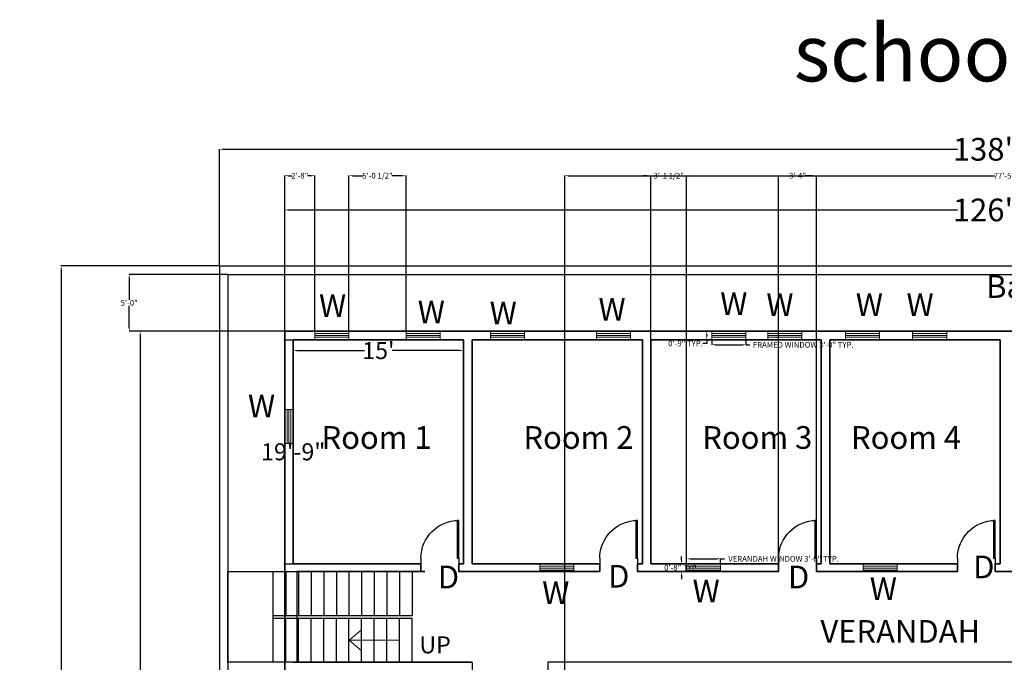
# Model space of a CAD drawing. Units: inches. Extents: x 6562 to 8578, y 2662 to 4218.
# Tile 2 of 3: x 6562 to 7603, y 3539 to 4218. Entities that reach past the tile are written whole.
import ezdxf

# ---------------------------------------------------------------- set-up
doc = ezdxf.new("R2010")
doc.units = ezdxf.units.IN
doc.header["$MEASUREMENT"] = 0
for name, color, linetype, lineweight in [('A-ANNO-DIMS', 2, 'Continuous', 18), ('A-ANNO-SYMB', 2, 'Continuous', 18), ('A-ANNO-TEXT', 7, 'Continuous', 18), ('A-AREA-IDEN', 7, 'Continuous', 25), ('A-DOOR', 3, 'Continuous', 25), ('A-FLOR-EDGE', 8, 'Continuous', 25), ('A-FLOR-STRS', 7, 'Continuous', 25), ('A-GLAZ', 4, 'Continuous', 18), ('A-WALL', 7, 'Continuous', 35)]:
    doc.layers.add(name, color=color, linetype=linetype, lineweight=lineweight)
doc.styles.get("Standard").update_dxf_attribs({"font": 'arial.ttf'})
doc.dimstyles.get("Standard").update_dxf_attribs({"dimtxt": 6, "dimasz": 4, "dimexe": 0.18, "dimexo": 0.0625, "dimgap": 0.09, "dimtad": 0, "dimtih": 1, "dimtoh": 1, "dimdec": 0, "dimzin": 0, "dimdsep": 46, "dimlunit": 3, "dimtxsty": 'Standard', "dimcen": 0.09, "dimadec": 0, "dimazin": 0, "dimtfac": 1, "dimtdec": 0, "dimtofl": 0, "dimtmove": 0, "dimatfit": 3, "dimfxl": 1, "dimtolj": 1, "dimtzin": 0, "dimarcsym": 0})

# ---------------------------------------------------------------- blocks, each defined once
blk = doc.blocks.new('*U8')
for p, q in [((0, 0), (0, -6)), ((40, 0), (40, -6))]:
    blk.add_line(p, q)
blk.add_lwpolyline([(0, 0), (0, 40), (1.75, 40), (1.75, 0)], close=True)
blk.add_arc((0, 0), 40, 0, 90)
blk = doc.blocks.new('*D11')
at = {"layer": 'A-ANNO-DIMS', "color": 0, "lineweight": -2, "transparency": 16777216}
for p, q in [((6773.2, 3958.1), (6773.2, 4081.4)), ((6777.2, 4081.2), (7553.2, 4081.2)), ((8428.2, 4081.2), (7652.2, 4081.2)), ((8432.2, 3958.1), (8432.2, 4081.4))]:
    blk.add_line(p, q, dxfattribs=at)
at = {"layer": 'A-ANNO-DIMS', "color": 0, "transparency": 16777216}
for points in [[(6777.2, 4081.9), (6777.2, 4080.6), (6773.2, 4081.2)], [(8428.2, 4081.9), (8428.2, 4080.6), (8432.2, 4081.2)]]:
    blk.add_solid(points, dxfattribs=at)
at = {"layer": 'Defpoints', "color": 0, "transparency": 16777216}
for p in [(8432.2, 4081.2), (6773.2, 3958), (8432.2, 3958)]:
    blk.add_point(p, dxfattribs=at)
at = {"layer": 'A-ANNO-DIMS', "color": 0, "transparency": 16777216, "insert": (7602.7, 4081.2), "char_height": 6, "attachment_point": 5}
blk.add_mtext('\\A1;{\\H4x;138\'-3"}', dxfattribs=at)
blk = doc.blocks.new('*D12')
at = {"layer": 'A-ANNO-DIMS', "color": 0, "lineweight": -2, "transparency": 16777216}
for p, q in [((6842.2, 3889.1), (6842.2, 4017.3)), ((6846.2, 4017.1), (7553.2, 4017.1)), ((8359.2, 4017.1), (7652.2, 4017.1)), ((8363.2, 3889.1), (8363.2, 4017.3))]:
    blk.add_line(p, q, dxfattribs=at)
at = {"layer": 'A-ANNO-DIMS', "color": 0, "transparency": 16777216}
for points in [[(6846.2, 4017.8), (6846.2, 4016.4), (6842.2, 4017.1)], [(8359.2, 4017.8), (8359.2, 4016.4), (8363.2, 4017.1)]]:
    blk.add_solid(points, dxfattribs=at)
at = {"layer": 'Defpoints', "color": 0, "transparency": 16777216}
for p in [(8363.2, 4017.1), (6842.2, 3889), (8363.2, 3889)]:
    blk.add_point(p, dxfattribs=at)
at = {"layer": 'A-ANNO-DIMS', "color": 0, "transparency": 16777216, "insert": (7602.7, 4017.1), "char_height": 6, "attachment_point": 5}
blk.add_mtext('\\A1;{\\H4x;126\'-9"}', dxfattribs=at)
blk = doc.blocks.new('*D13')
at = {"layer": 'A-ANNO-DIMS', "color": 0, "lineweight": -2, "transparency": 16777216}
for p, q in [((6773.1, 3958), (6605.8, 3958)), ((6606, 3954), (6606, 3371.8)), ((6606, 2765), (6606, 3347.2)), ((6773.1, 2761), (6605.8, 2761))]:
    blk.add_line(p, q, dxfattribs=at)
at = {"layer": 'A-ANNO-DIMS', "color": 0, "transparency": 16777216}
for points in [[(6605.3, 3954), (6606.6, 3954), (6606, 3958)], [(6605.3, 2765), (6606.6, 2765), (6606, 2761)]]:
    blk.add_solid(points, dxfattribs=at)
at = {"layer": 'Defpoints', "color": 0, "transparency": 16777216}
for p in [(6773.2, 3958), (6606, 2761), (6773.2, 2761)]:
    blk.add_point(p, dxfattribs=at)
at = {"layer": 'A-ANNO-DIMS', "color": 0, "transparency": 16777216, "insert": (6606, 3359.5), "char_height": 6, "attachment_point": 5}
blk.add_mtext('\\A1;{\\H4x;99\'-9"}', dxfattribs=at)
blk = doc.blocks.new('*D14')
at = {"layer": 'A-ANNO-DIMS', "color": 0, "lineweight": -2, "transparency": 16777216}
for p, q in [((6842.1, 3889), (6689.3, 3889)), ((6689.4, 3885), (6689.4, 3337.3)), ((6689.4, 2765), (6689.4, 3312.7)), ((6842.1, 2761), (6689.3, 2761))]:
    blk.add_line(p, q, dxfattribs=at)
at = {"layer": 'A-ANNO-DIMS', "color": 0, "transparency": 16777216}
for points in [[(6688.8, 3885), (6690.1, 3885), (6689.4, 3889)], [(6688.8, 2765), (6690.1, 2765), (6689.4, 2761)]]:
    blk.add_solid(points, dxfattribs=at)
at = {"layer": 'Defpoints', "color": 0, "transparency": 16777216}
for p in [(6842.2, 3889), (6689.4, 2761), (6842.2, 2761)]:
    blk.add_point(p, dxfattribs=at)
at = {"layer": 'A-ANNO-DIMS', "color": 0, "transparency": 16777216, "insert": (6689.4, 3325), "char_height": 6, "attachment_point": 5}
blk.add_mtext("\\A1;{\\H4x;94'}", dxfattribs=at)
blk = doc.blocks.new('*D27')
at = {"layer": 'A-ANNO-DIMS', "color": 0, "lineweight": -2, "transparency": 16777216}
for p, q in [((6841.2, 3880), (6851.4, 3880)), ((6851.2, 3876), (6851.2, 3770.8)), ((6851.2, 3647), (6851.2, 3752.2)), ((6841.2, 3643), (6851.4, 3643))]:
    blk.add_line(p, q, dxfattribs=at)
at = {"layer": 'A-ANNO-DIMS', "color": 0, "transparency": 16777216}
for points in [[(6850.5, 3876), (6851.8, 3876), (6851.2, 3880)], [(6850.5, 3647), (6851.8, 3647), (6851.2, 3643)]]:
    blk.add_solid(points, dxfattribs=at)
at = {"layer": 'Defpoints', "color": 0, "transparency": 16777216}
for p in [(6841.1, 3880), (6851.2, 3880), (6841.1, 3643)]:
    blk.add_point(p, dxfattribs=at)
at = {"layer": 'A-ANNO-DIMS', "color": 0, "transparency": 16777216, "insert": (6851.2, 3761.5), "char_height": 6, "attachment_point": 5}
blk.add_mtext('\\A1;{\\H3x;19\'-9"}', dxfattribs=at)
blk = doc.blocks.new('*D28')
at = {"layer": 'A-ANNO-DIMS', "color": 0, "lineweight": -2, "transparency": 16777216}
for p, q in [((6851.2, 3879.9), (6851.2, 3868.3)), ((7031.2, 3879.9), (7031.2, 3868.3)), ((6855.2, 3868.5), (6926.7, 3868.5)), ((7027.2, 3868.5), (6955.7, 3868.5))]:
    blk.add_line(p, q, dxfattribs=at)
at = {"layer": 'A-ANNO-DIMS', "color": 0, "transparency": 16777216}
for points in [[(6855.2, 3869.2), (6855.2, 3867.8), (6851.2, 3868.5)], [(7027.2, 3869.2), (7027.2, 3867.8), (7031.2, 3868.5)]]:
    blk.add_solid(points, dxfattribs=at)
at = {"layer": 'Defpoints', "color": 0, "transparency": 16777216}
for p in [(6851.2, 3880), (7031.2, 3880), (7031.2, 3868.5)]:
    blk.add_point(p, dxfattribs=at)
at = {"layer": 'A-ANNO-DIMS', "color": 0, "transparency": 16777216, "insert": (6941.2, 3868.5), "char_height": 6, "attachment_point": 5}
blk.add_mtext("\\A1;{\\H3x;15'}", dxfattribs=at)
blk = doc.blocks.new('WIN-36-FRAMED')
for p, q in [((2.5, 36), (2.5, 0)), ((4.5, 36), (4.5, 0)), ((6.5, 36), (6.5, 0))]:
    blk.add_line(p, q)
blk.add_lwpolyline([(0, 36), (9, 36), (9, 0), (0, 0)], close=True)
blk = doc.blocks.new('STAIR-HALF-TURN')
for p, q in [((0, 96), (194.7, 96)), ((0, 96), (0, 49.3)), ((13.3, 96), (13.3, 49.3)), ((26.7, 96), (26.7, 49.3)), ((40, 96), (40, 49.3)), ((53.3, 96), (53.3, 49.3)), ((66.7, 96), (66.7, 49.3)), ((80, 96), (80, 49.3)), ((93.3, 96), (93.3, 49.3)), ((106.7, 96), (106.7, 49.3)), ((120, 96), (120, 49.3)), ((133.3, 96), (133.3, 49.3)), ((146.7, 96), (146.7, 48)), ((194.7, 96), (194.7, 48)), ((146.7, 49.3), (0, 49.3)), ((0, 0), (0, 46.7)), ((146.7, 46.7), (0, 46.7)), ((13.3, 0), (13.3, 46.7)), ((26.7, 0), (26.7, 46.7)), ((40, 0), (40, 46.7)), ((53.3, 0), (53.3, 46.7)), ((66.7, 0), (66.7, 46.7)), ((80, 0), (80, 46.7)), ((93.3, 0), (93.3, 46.7)), ((106.7, 0), (106.7, 46.7)), ((120, 0), (120, 46.7)), ((133.3, 0), (133.3, 46.7)), ((146.7, 48), (146.7, 0)), ((194.7, 48), (194.7, 0)), ((194.7, 0), (0, 0))]:
    blk.add_line(p, q)
blk = doc.blocks.new('WIN-36-VERANDA')
for p, q in [((0, 0), (0, 7.9)), ((36, 5.5), (0, 5.5)), ((36, 3.5), (0, 3.5)), ((36, 1.5), (0, 1.5)), ((36, 8), (36, 0))]:
    blk.add_line(p, q)
blk = doc.blocks.new('ARROW-STAIR-UP')
for p, q in [((0, 11.1), (13.3, 22.2)), ((53.3, 11.1), (0, 11.1)), ((0, 11.1), (13.3, 0))]:
    blk.add_line(p, q)
blk = doc.blocks.new('WIN-36-OFFSET')
for p, q in [((2.5, 36), (2.5, 0)), ((4.5, 36), (4.5, 0)), ((6.5, 36), (6.5, 0))]:
    blk.add_line(p, q)
blk.add_lwpolyline([(0, 36), (9, 36), (9, 0), (0, 0)], close=True)
blk = doc.blocks.new('*D35')
at = {"layer": 'A-ANNO-DIMS', "color": 0, "lineweight": -2, "transparency": 16777216}
for p, q in [((7293.6, 3879.9), (7293.6, 3874.4)), ((7297.6, 3874.6), (7325.6, 3874.6)), ((7329.6, 3879.9), (7329.6, 3874.4)), ((7329.6, 3874.6), (7333.6, 3874.6))]:
    blk.add_line(p, q, dxfattribs=at)
at = {"layer": 'A-ANNO-DIMS', "color": 0, "transparency": 16777216}
for points in [[(7297.6, 3875.3), (7297.6, 3873.9), (7293.6, 3874.6)], [(7325.6, 3875.3), (7325.6, 3873.9), (7329.6, 3874.6)]]:
    blk.add_solid(points, dxfattribs=at)
at = {"layer": 'Defpoints', "color": 0, "transparency": 16777216}
for p in [(7293.6, 3880), (7329.6, 3880), (7329.6, 3874.6)]:
    blk.add_point(p, dxfattribs=at)
at = {"layer": 'A-ANNO-DIMS', "color": 0, "transparency": 16777216, "insert": (7390.2, 3874.6), "char_height": 6, "attachment_point": 5}
blk.add_mtext('\\A1;FRAMED WINDOW 3\'-0" TYP.', dxfattribs=at)
blk = doc.blocks.new('*D36')
at = {"layer": 'A-ANNO-DIMS', "color": 0, "lineweight": -2, "transparency": 16777216}
for p, q in [((7293.5, 3889), (7288, 3889)), ((7288.2, 3885), (7288.2, 3884)), ((7288.2, 3876), (7284.2, 3876)), ((7293.5, 3880), (7288, 3880)), ((7288.2, 3880), (7288.2, 3876))]:
    blk.add_line(p, q, dxfattribs=at)
at = {"layer": 'A-ANNO-DIMS', "color": 0, "transparency": 16777216}
for points in [[(7287.5, 3885), (7288.8, 3885), (7288.2, 3889)], [(7287.5, 3884), (7288.8, 3884), (7288.2, 3880)]]:
    blk.add_solid(points, dxfattribs=at)
at = {"layer": 'Defpoints', "color": 0, "transparency": 16777216}
for p in [(7293.6, 3889), (7288.2, 3880), (7293.6, 3880)]:
    blk.add_point(p, dxfattribs=at)
at = {"layer": 'A-ANNO-DIMS', "color": 0, "transparency": 16777216, "insert": (7265.8, 3876), "char_height": 6, "attachment_point": 5}
blk.add_mtext('\\A1;0\'-9" TYP.', dxfattribs=at)
blk = doc.blocks.new('*D39')
at = {"layer": 'A-ANNO-DIMS', "color": 0, "lineweight": -2, "transparency": 16777216}
for p, q in [((7266.9, 3643.1), (7266.9, 3648.6)), ((7270.9, 3648.4), (7298.9, 3648.4)), ((7302.9, 3643.1), (7302.9, 3648.6)), ((7302.9, 3648.4), (7306.9, 3648.4))]:
    blk.add_line(p, q, dxfattribs=at)
at = {"layer": 'A-ANNO-DIMS', "color": 0, "transparency": 16777216}
for points in [[(7270.9, 3649.1), (7270.9, 3647.7), (7266.9, 3648.4)], [(7298.9, 3649.1), (7298.9, 3647.7), (7302.9, 3648.4)]]:
    blk.add_solid(points, dxfattribs=at)
at = {"layer": 'Defpoints', "color": 0, "transparency": 16777216}
for p in [(7266.9, 3643), (7302.9, 3648.4), (7302.9, 3643)]:
    blk.add_point(p, dxfattribs=at)
at = {"layer": 'A-ANNO-DIMS', "color": 0, "transparency": 16777216, "insert": (7369.4, 3648.4), "char_height": 6, "attachment_point": 5}
blk.add_mtext('\\A1;VERANDAH WINDOW 3\'-0" TYP.', dxfattribs=at)
blk = doc.blocks.new('*D40')
at = {"layer": 'A-ANNO-DIMS', "color": 0, "lineweight": -2, "transparency": 16777216}
for p, q in [((7266.8, 3643), (7261.3, 3643)), ((7261.5, 3647), (7261.5, 3651)), ((7266.8, 3635), (7261.3, 3635)), ((7261.5, 3631), (7261.5, 3627))]:
    blk.add_line(p, q, dxfattribs=at)
at = {"layer": 'A-ANNO-DIMS', "color": 0, "transparency": 16777216}
for points in [[(7260.8, 3647), (7262.2, 3647), (7261.5, 3643)], [(7260.8, 3631), (7262.2, 3631), (7261.5, 3635)]]:
    blk.add_solid(points, dxfattribs=at)
at = {"layer": 'Defpoints', "color": 0, "transparency": 16777216}
for p in [(7261.5, 3643), (7266.9, 3643), (7266.9, 3635)]:
    blk.add_point(p, dxfattribs=at)
at = {"layer": 'A-ANNO-DIMS', "color": 0, "transparency": 16777216, "insert": (7261.5, 3639), "char_height": 6, "attachment_point": 5}
blk.add_mtext('\\A1;0\'-8" TYP.', dxfattribs=at)
blk = doc.blocks.new('*D45')
at = {"layer": 'A-ANNO-DIMS', "color": 0, "lineweight": -2, "transparency": 16777216}
for p, q in [((7138.2, 2935.1), (7138.2, 4053.4)), ((7142.2, 4053.3), (7592.3, 4053.3)), ((8063.2, 4053.3), (7613, 4053.3)), ((8067.2, 3057.1), (8067.2, 4053.4))]:
    blk.add_line(p, q, dxfattribs=at)
at = {"layer": 'A-ANNO-DIMS', "color": 0, "transparency": 16777216}
for points in [[(7142.2, 4053.9), (7142.2, 4052.6), (7138.2, 4053.3)], [(8063.2, 4053.9), (8063.2, 4052.6), (8067.2, 4053.3)]]:
    blk.add_solid(points, dxfattribs=at)
at = {"layer": 'Defpoints', "color": 0, "transparency": 16777216}
for p in [(8067.2, 4053.3), (8067.2, 3057), (7138.2, 2935)]:
    blk.add_point(p, dxfattribs=at)
at = {"layer": 'A-ANNO-DIMS', "color": 0, "transparency": 16777216, "insert": (7602.7, 4053.3), "char_height": 6, "attachment_point": 5}
blk.add_mtext('\\A1;77\'-5"', dxfattribs=at)
blk = doc.blocks.new('*D47')
at = {"layer": 'A-ANNO-DIMS', "color": 0, "lineweight": -2, "transparency": 16777216}
for p, q in [((7040.2, 3538.9), (7040.2, 2665.6)), ((7120.2, 3538.9), (7120.2, 2665.6)), ((7044.2, 2665.8), (7072.1, 2665.8)), ((7116.2, 2665.8), (7088.3, 2665.8))]:
    blk.add_line(p, q, dxfattribs=at)
at = {"layer": 'A-ANNO-DIMS', "color": 0, "transparency": 16777216}
for points in [[(7044.2, 2666.4), (7044.2, 2665.1), (7040.2, 2665.8)], [(7116.2, 2666.4), (7116.2, 2665.1), (7120.2, 2665.8)]]:
    blk.add_solid(points, dxfattribs=at)
at = {"layer": 'Defpoints', "color": 0, "transparency": 16777216}
for p in [(7040.2, 3539), (7120.2, 3539), (7120.2, 2665.8)]:
    blk.add_point(p, dxfattribs=at)
at = {"layer": 'A-ANNO-DIMS', "color": 0, "transparency": 16777216, "insert": (7080.2, 2665.8), "char_height": 6, "attachment_point": 5}
blk.add_mtext('\\A1;6\'-8"', dxfattribs=at)
blk = doc.blocks.new('*D50')
at = {"layer": 'A-ANNO-DIMS', "color": 0, "lineweight": -2, "transparency": 16777216}
for p, q in [((7364.2, 3643.1), (7364.2, 4053.4)), ((7368.2, 4053.3), (7376.1, 4053.3)), ((7400.2, 4053.3), (7392.2, 4053.3)), ((7404.2, 3643.1), (7404.2, 4053.4))]:
    blk.add_line(p, q, dxfattribs=at)
at = {"layer": 'A-ANNO-DIMS', "color": 0, "transparency": 16777216}
for points in [[(7368.2, 4053.9), (7368.2, 4052.6), (7364.2, 4053.3)], [(7400.2, 4053.9), (7400.2, 4052.6), (7404.2, 4053.3)]]:
    blk.add_solid(points, dxfattribs=at)
at = {"layer": 'Defpoints', "color": 0, "transparency": 16777216}
for p in [(7404.2, 4053.3), (7364.2, 3643), (7404.2, 3643)]:
    blk.add_point(p, dxfattribs=at)
at = {"layer": 'A-ANNO-DIMS', "color": 0, "transparency": 16777216, "insert": (7384.2, 4053.3), "char_height": 6, "attachment_point": 5}
blk.add_mtext('\\A1;3\'-4"', dxfattribs=at)
blk = doc.blocks.new('*D52')
at = {"layer": 'A-ANNO-DIMS', "color": 0, "lineweight": -2, "transparency": 16777216}
for p, q in [((6842.2, 3889.1), (6842.2, 4053.4)), ((6846.2, 4053.3), (6850, 4053.3)), ((6870.1, 4053.3), (6866.3, 4053.3)), ((6874.1, 3889.1), (6874.1, 4053.4))]:
    blk.add_line(p, q, dxfattribs=at)
at = {"layer": 'A-ANNO-DIMS', "color": 0, "transparency": 16777216}
for points in [[(6846.2, 4053.9), (6846.2, 4052.6), (6842.2, 4053.3)], [(6870.1, 4053.9), (6870.1, 4052.6), (6874.1, 4053.3)]]:
    blk.add_solid(points, dxfattribs=at)
at = {"layer": 'Defpoints', "color": 0, "transparency": 16777216}
for p in [(6874.1, 4053.3), (6842.2, 3889), (6874.1, 3889)]:
    blk.add_point(p, dxfattribs=at)
at = {"layer": 'A-ANNO-DIMS', "color": 0, "transparency": 16777216, "insert": (6858.1, 4053.3), "char_height": 6, "attachment_point": 5}
blk.add_mtext('\\A1;2\'-8"', dxfattribs=at)
blk = doc.blocks.new('*D53')
at = {"layer": 'A-ANNO-DIMS', "color": 0, "lineweight": -2, "transparency": 16777216}
for p, q in [((6910.1, 3889.1), (6910.1, 4053.4)), ((6914.1, 4053.3), (6925.2, 4053.3)), ((6966.4, 4053.3), (6955.3, 4053.3)), ((6970.4, 3889.1), (6970.4, 4053.4))]:
    blk.add_line(p, q, dxfattribs=at)
at = {"layer": 'A-ANNO-DIMS', "color": 0, "transparency": 16777216}
for points in [[(6914.1, 4053.9), (6914.1, 4052.6), (6910.1, 4053.3)], [(6966.4, 4053.9), (6966.4, 4052.6), (6970.4, 4053.3)]]:
    blk.add_solid(points, dxfattribs=at)
at = {"layer": 'Defpoints', "color": 0, "transparency": 16777216}
for p in [(6970.4, 4053.3), (6910.1, 3889), (6970.4, 3889)]:
    blk.add_point(p, dxfattribs=at)
at = {"layer": 'A-ANNO-DIMS', "color": 0, "transparency": 16777216, "insert": (6940.3, 4053.3), "char_height": 6, "attachment_point": 5}
blk.add_mtext('\\A1;5\'-0 1/2"', dxfattribs=at)
blk = doc.blocks.new('*D54')
at = {"layer": 'A-ANNO-DIMS', "color": 0, "lineweight": -2, "transparency": 16777216}
for p, q in [((6782.1, 3949), (6677.7, 3949)), ((6677.9, 3945), (6677.9, 3922.2)), ((6677.9, 3893), (6677.9, 3915.8)), ((6842.1, 3889), (6677.7, 3889))]:
    blk.add_line(p, q, dxfattribs=at)
at = {"layer": 'A-ANNO-DIMS', "color": 0, "transparency": 16777216}
for points in [[(6677.3, 3945), (6678.6, 3945), (6677.9, 3949)], [(6677.3, 3893), (6678.6, 3893), (6677.9, 3889)]]:
    blk.add_solid(points, dxfattribs=at)
at = {"layer": 'Defpoints', "color": 0, "transparency": 16777216}
for p in [(6782.2, 3949), (6677.9, 3889), (6842.2, 3889)]:
    blk.add_point(p, dxfattribs=at)
at = {"layer": 'A-ANNO-DIMS', "color": 0, "transparency": 16777216, "insert": (6677.9, 3919), "char_height": 6, "attachment_point": 5}
blk.add_mtext('\\A1;5\'-0"', dxfattribs=at)
blk = doc.blocks.new('*D59')
at = {"layer": 'A-ANNO-DIMS', "color": 0, "lineweight": -2, "transparency": 16777216}
for p, q in [((7225.2, 4053.3), (7221.2, 4053.3)), ((7229.2, 3643.1), (7229.2, 4053.4)), ((7266.9, 3643), (7266.9, 4053.4)), ((7270.9, 4053.3), (7274.9, 4053.3))]:
    blk.add_line(p, q, dxfattribs=at)
at = {"layer": 'A-ANNO-DIMS', "color": 0, "transparency": 16777216}
for points in [[(7225.2, 4053.9), (7225.2, 4052.6), (7229.2, 4053.3)], [(7270.9, 4053.9), (7270.9, 4052.6), (7266.9, 4053.3)]]:
    blk.add_solid(points, dxfattribs=at)
at = {"layer": 'Defpoints', "color": 0, "transparency": 16777216}
for p in [(7266.9, 4053.3), (7229.2, 3643), (7266.9, 3642.9)]:
    blk.add_point(p, dxfattribs=at)
at = {"layer": 'A-ANNO-DIMS', "color": 0, "transparency": 16777216, "insert": (7248, 4053.3), "char_height": 6, "attachment_point": 5}
blk.add_mtext('\\A1;3\'-1 1/2"', dxfattribs=at)

msp = doc.modelspace()

# ---------------------------------------------------------------- linework, layer by layer
at = {"layer": 'A-ANNO-SYMB'}
msp.add_line((6963.51, 3562.34), (6963.51, 3562.34), dxfattribs=at)
at = {"layer": 'A-FLOR-EDGE'}
for p, q in [((6773.18, 3958), (6773.18, 2761)), ((6773.18, 3958), (8432.18, 3958)), ((6782.18, 3949), (6782.18, 2770)), ((6782.18, 3949), (8423.18, 3949)), ((8085.18, 3539), (7120.18, 3539))]:
    msp.add_line(p, q, dxfattribs=at)
at = {"layer": 'A-FLOR-STRS'}
msp.add_line((6855.18, 3635), (6855.18, 3539), dxfattribs=at)
at = {"layer": 'A-GLAZ'}
msp.add_line((6892.66, 3643), (6928.66, 3643), dxfattribs=at)
at = {"layer": 'A-WALL'}
for p, q in [((6842.18, 3889), (8363.18, 3889)), ((6842.18, 3889), (6842.18, 2770)), ((6851.18, 3880), (7031.18, 3880)), ((6851.18, 3880), (6851.18, 3643)), ((7031.18, 3880), (7031.18, 3643)), ((7040.18, 3880), (7040.18, 3643)), ((7040.18, 3880), (7220.18, 3880)), ((7220.18, 3880), (7220.18, 3643)), ((7229.18, 3880), (7229.18, 3643)), ((7229.18, 3880), (7409.18, 3880)), ((7409.18, 3880), (7409.18, 3643)), ((7418.18, 3880), (7418.18, 3643)), ((7418.18, 3880), (7598.18, 3880)), ((7598.18, 3880), (7598.18, 3643)), ((6986.18, 3643), (6851.18, 3643)), ((6986.18, 3643), (6986.18, 3635)), ((7031.18, 3643), (7026.18, 3643)), ((7026.18, 3643), (7026.18, 3635)), ((7175.18, 3643), (7040.18, 3643)), ((7175.18, 3643), (7175.18, 3635)), ((7220.18, 3643), (7215.18, 3643)), ((7215.18, 3643), (7215.18, 3635)), ((7220.18, 3643), (7220.18, 3643)), ((7364.18, 3643), (7229.18, 3643)), ((7364.18, 3643), (7364.18, 3635)), ((7409.18, 3643), (7404.18, 3643)), ((7404.18, 3643), (7404.18, 3635)), ((7553.18, 3643), (7418.18, 3643)), ((7553.18, 3643), (7553.18, 3635)), ((7598.18, 3643), (7593.18, 3643)), ((7593.18, 3643), (7593.18, 3635)), ((6990.18, 3635), (6855.18, 3635)), ((7175.18, 3635), (7026.18, 3635)), ((7031.18, 3635), (7031.18, 3635)), ((7364.18, 3635), (7215.18, 3635)), ((7553.18, 3635), (7404.18, 3635)), ((7409.18, 3635), (7409.18, 3635)), ((7742.18, 3635), (7593.18, 3635)), ((7040.18, 3539), (6851.18, 3539))]:
    msp.add_line(p, q, dxfattribs=at)

# ---------------------------------------------------------------- block references
at = {"layer": 'A-ANNO-SYMB'}
msp.add_blockref('ARROW-STAIR-UP', (6910.18, 3551.22), dxfattribs=at)
at = {"layer": 'A-DOOR', "xscale": -1}
for p in [(7026.18, 3649), (7215.18, 3649), (7404.18, 3649), (7593.18, 3649)]:
    msp.add_blockref('*U8', p, dxfattribs=at)
at = {"layer": 'A-FLOR-STRS', "rotation": 180}
msp.add_blockref('STAIR-HALF-TURN', (6976.84, 3635), dxfattribs=at)
at = {"layer": 'A-GLAZ'}
for p, rotation in [((6874.1, 3889), 270.0000000000009), ((6970.4, 3889), 270.0000000000009), ((7059.53, 3889), 270.0000000000028), ((7059.53, 3889), 270.0000000000028), ((7171.56, 3889), 270.0000000000015), ((7293.56, 3889), 270.0000000000009), ((7352.66, 3889), 270.0000000000009), ((7434.95, 3889), 270.0000000000015), ((7505.81, 3889), 269.9999999999997), ((7505.81, 3889), 269.9999999999997)]:
    msp.add_blockref('WIN-36-FRAMED', p, dxfattribs=dict(at, rotation=rotation))
for name, p in [('WIN-36-OFFSET', (6842.18, 3770.3)), ('WIN-36-VERANDA', (7111.9, 3635)), ('WIN-36-VERANDA', (7266.89, 3635)), ('WIN-36-VERANDA', (7453.56, 3635))]:
    msp.add_blockref(name, p, dxfattribs=at)

# ---------------------------------------------------------------- texts
at = {"layer": 'A-ANNO-TEXT', "attachment_point": 1}
for s, width, insert, char_height in [('school layout plan', 1424.8444, (7380.26, 4213.03), 60), ('W', 32.1856, (6878.45, 3928.04), 24), ('W', 32.1856, (7173.77, 3924.15), 24), ('W', 32.1856, (7302.43, 3929.99), 24), ('W', 32.1856, (7351.16, 3929.01), 24), ('W', 32.1856, (7445.71, 3929.01), 24), ('W', 32.1856, (7499.31, 3929.01), 24), ('W', 32.1856, (6982.74, 3921.23), 24), ('W', 32.1856, (7058.76, 3920.25), 24), ('W', 32.1856, (6803.4, 3821.93), 24), ('D', 32.1856, (7183.97, 3641.98), 24), ('D', 32.1856, (7569.76, 3651.83), 24), ('D', 32.1856, (7003.95, 3641.15), 24), ('D', 32.1856, (7373.99, 3641.15), 24), ('W', 32.1856, (7114.32, 3624.48), 24), ('W', 32.1856, (7273.22, 3626.34), 24), ('W', 32.1856, (7460.49, 3628.73), 24), ('UP', 38.7631, (6984.54, 3566.43), 18)]:
    msp.add_mtext_dynamic_manual_height_columns(s, width=width, gutter_width=40, heights=[0], dxfattribs=dict(at, insert=insert, char_height=char_height))
at = {"layer": 'A-AREA-IDEN', "char_height": 24, "attachment_point": 1}
for s, width, gutter_width, insert in [('Balcony', 33.181, 40, (7583.46, 3948.18)), ('Room 1', 125.7129, 1, (6881.11, 3788.61)), ('Room 2', 125.7129, 1, (7094.46, 3788.61)), ('Room 3', 125.7129, 1, (7283.46, 3788.61)), ('Room 4', 125.7129, 1, (7440.68, 3788.61)), ('VERANDAH', 211.1035, 40, (7408.33, 3583.65))]:
    msp.add_mtext_dynamic_manual_height_columns(s, width=width, gutter_width=gutter_width, heights=[0], dxfattribs=dict(at, insert=insert))

# ---------------------------------------------------------------- dimensions: what is measured, and where the dimension line sits
at = {"layer": 'A-ANNO-DIMS'}
for base, p1, p2, text, override, picture, middle in [((8432.18, 4081.22), (6773.18, 3958), (8432.18, 3958), '{\\H4x;<>}', {"dimclrd": 0, "dimclre": 0, "dimclrt": 0}, '*D11', (7602.68, 4081.22)), ((8363.18, 4017.09), (6842.18, 3889), (8363.18, 3889), '{\\H4x;<>}', {"dimclrd": 0, "dimclre": 0, "dimclrt": 0}, '*D12', (7602.68, 4017.09)), ((7031.18, 3868.48), (6851.18, 3880), (7031.18, 3880), '{\\H3x;<>}', {"dimclrd": 0, "dimclre": 0, "dimclrt": 0}, '*D28', (6941.18, 3868.48)), ((7302.89, 3648.4), (7266.89, 3643), (7302.89, 3643), 'VERANDAH WINDOW <> TYP.', {"dimdec": 1, "dimlfac": 1, "dimrnd": 0, "dimzin": 1, "dimdsep": 46, "dimlunit": 4, "dimfrac": 2}, '*D39', (7369.43, 3648.4))]:
    dim = msp.add_linear_dim(base=base, p1=p1, p2=p2, text=text, dimstyle='Standard', override=override, dxfattribs=at)
    dim.commit()
    dim.dimension.update_dxf_attribs({"geometry": picture, "text_midpoint": middle})
for base, p1, p2, picture, middle in [((6970.4, 4053.25), (6910.1, 3889), (6970.4, 3889), '*D53', (6940.25, 4053.25)), ((7266.89, 4053.25), (7229.18, 3643), (7266.89, 3642.93), '*D59', (7248.04, 4053.25)), ((6874.1, 4053.25), (6842.18, 3889), (6874.1, 3889), '*D52', (6858.14, 4053.25)), ((8067.18, 4053.25), (7138.17, 2935), (8067.18, 3057), '*D45', (7602.68, 4053.25)), ((7404.18, 4053.25), (7364.18, 3643), (7404.18, 3643), '*D50', (7384.18, 4053.25)), ((7120.18, 2665.75), (7040.18, 3539), (7120.18, 3539), '*D47', (7080.18, 2665.75))]:
    dim = msp.add_linear_dim(base=base, p1=p1, p2=p2, dimstyle='Standard', override={"dimdec": 1, "dimlfac": 1, "dimrnd": 0, "dimzin": 1, "dimdsep": 46, "dimlunit": 4, "dimfrac": 2}, dxfattribs=at)
    dim.commit()
    dim.dimension.update_dxf_attribs({"geometry": picture, "text_midpoint": middle})
for base, p1, p2, angle, text, override, picture, middle in [((6605.96, 2761), (6773.18, 3958), (6773.18, 2761), 90, '{\\H4x;<>}', {"dimclrd": 0, "dimclre": 0, "dimclrt": 0}, '*D13', (6605.96, 3359.5)), ((7329.56, 3874.6), (7293.56, 3880), (7329.56, 3880), 0, 'FRAMED WINDOW <> TYP.', {"dimdec": 1, "dimlfac": 1, "dimrnd": 0, "dimzin": 1, "dimdsep": 46, "dimlunit": 4, "dimfrac": 2}, '*D35', (7390.18, 3874.6)), ((6689.45, 2761), (6842.18, 3889), (6842.18, 2761), 90, '{\\H4x;<>}', {"dimclrd": 0, "dimclre": 0, "dimclrt": 0}, '*D14', (6689.45, 3325)), ((7288.16, 3880), (7293.56, 3889), (7293.56, 3880), 270, '<> TYP.', {"dimdec": 1, "dimlfac": 1, "dimrnd": 0, "dimzin": 1, "dimdsep": 46, "dimlunit": 4, "dimfrac": 2}, '*D36', (7265.78, 3876)), ((6851.18, 3880), (6841.14, 3643), (6841.14, 3880), 90, '{\\H3x;<>}', {"dimclrd": 0, "dimclre": 0, "dimclrt": 0}, '*D27', (6851.18, 3761.5)), ((7261.49, 3643), (7266.89, 3635), (7266.89, 3643), 90, '<> TYP.', {"dimdec": 1, "dimlfac": 1, "dimrnd": 0, "dimzin": 1, "dimdsep": 46, "dimlunit": 4, "dimfrac": 2}, '*D40', (7261.49, 3639))]:
    dim = msp.add_linear_dim(base=base, p1=p1, p2=p2, angle=angle, text=text, dimstyle='Standard', override=override, dxfattribs=at)
    dim.commit()
    dim.dimension.update_dxf_attribs({"geometry": picture, "text_midpoint": middle})
dim = msp.add_linear_dim(base=(6677.93, 3889), p1=(6782.18, 3949), p2=(6842.18, 3889), angle=90, dimstyle='Standard', override={"dimdec": 1, "dimlfac": 1, "dimrnd": 0, "dimzin": 1, "dimdsep": 46, "dimlunit": 4, "dimfrac": 2}, dxfattribs=at)
dim.commit()
dim.dimension.update_dxf_attribs({"geometry": '*D54', "text_midpoint": (6677.93, 3919)})

doc.saveas('drawing.dxf')
